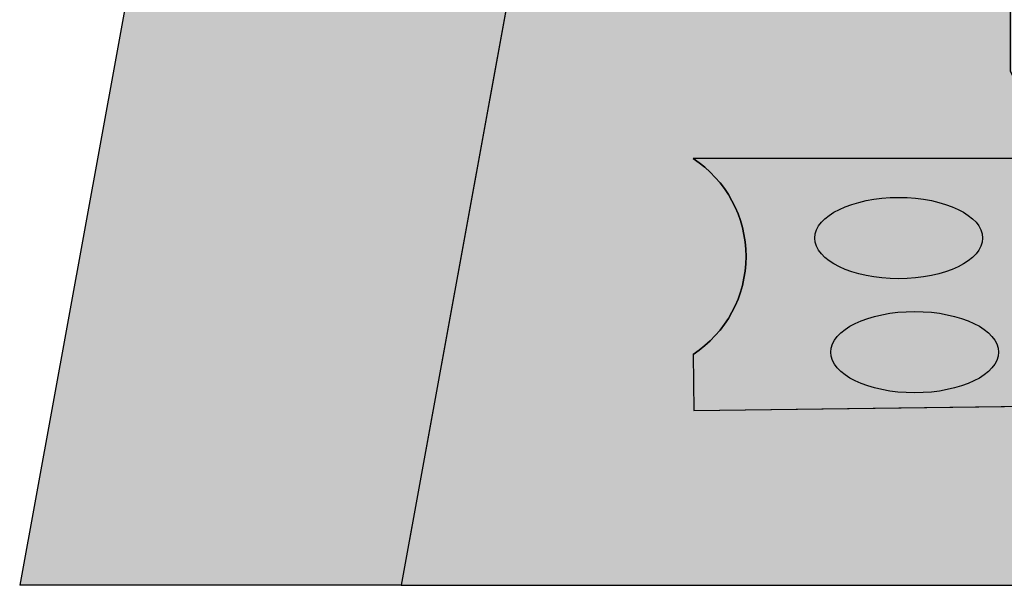
# Model space of a CAD drawing. Units: feet. Extents: x 3168 to 4724, y 827 to 1477.
# Tile 1 of 256: x 3168 to 3599, y 827 to 1075. Entities that reach past the tile are written whole.
import ezdxf

# ---------------------------------------------------------------- set-up
doc = ezdxf.new("R2010")
doc.units = ezdxf.units.FT
doc.layers.add('A-ELEV-PATT', color=8, linetype='Continuous', lineweight=13)
doc.layers.add('C-TOPO', color=3, linetype='Continuous', lineweight=25)

msp = doc.modelspace()

# ---------------------------------------------------------------- hatches: boundary and pattern name
at = {"layer": 'A-ELEV-PATT'}
h = msp.add_hatch(color=256, dxfattribs=at)
h.dxf.hatch_style = 1
edge = h.paths.add_edge_path()
edge.add_ellipse((3552.91, 979.22), major_axis=(36.74, 0), ratio=0.484848, start_angle=0, end_angle=360)
edge = h.paths.add_edge_path()
edge.add_ellipse((3559.89, 929.25), major_axis=(36.74, 0), ratio=0.484848, start_angle=0, end_angle=360)
edge = h.paths.add_edge_path()
edge.add_line((3299.32, 1198.61), (3479.92, 1198.61))
edge.add_line((3479.92, 1198.61), (3479.92, 1209.87))
edge.add_spline(control_points=[(3479.92, 1209.87), (3464.3, 1209.87), (3448.69, 1209.87), (3410.95, 1209.87), (3388.83, 1209.87), (3355.65, 1209.87), (3344.59, 1209.87), (3328, 1209.87), (3322.47, 1209.87), (3314.17, 1209.87), (3311.41, 1209.87), (3307.26, 1209.87), (3305.87, 1209.87), (3303.8, 1209.87), (3303.11, 1209.87), (3302.07, 1209.87), (3301.73, 1209.87), (3301.21, 1209.87), (3301.04, 1209.87), (3300.78, 1209.87), (3300.69, 1209.87), (3300.56, 1209.87), (3300.52, 1209.87), (3300.45, 1209.87), (3300.43, 1209.87), (3300.4, 1209.87), (3300.39, 1209.87), (3300.37, 1209.87), (3300.35, 1209.87), (3300.35, 1209.87), (3300.35, 1209.87), (3300.34, 1209.87), (3300.34, 1209.87), (3300.34, 1209.87), (3300.34, 1209.87), (3300.33, 1209.87), (3300.33, 1209.87), (3300.33, 1209.87), (3300.32, 1209.87), (3300.31, 1209.87), (3300.31, 1209.87), (3300.29, 1209.87), (3300.28, 1209.87), (3300.23, 1209.87), (3300.2, 1209.87), (3299.95, 1209.87), (3299.74, 1209.87), (3299.44, 1209.88), (3299.33, 1209.89), (3299.18, 1209.89), (3299.13, 1209.9), (3298.65, 1209.92), (3298.23, 1209.95), (3297.6, 1210), (3297.39, 1210.02), (3297.08, 1210.06), (3296.98, 1210.07), (3296.29, 1210.15), (3295.72, 1210.24), (3294.87, 1210.4), (3294.59, 1210.45), (3294.17, 1210.54), (3294.03, 1210.57), (3291.71, 1211.1), (3289.65, 1211.81), (3285.78, 1213.56), (3283.95, 1214.6), (3280.51, 1216.98), (3278.9, 1218.32), (3276.38, 1220.83), (3275.42, 1221.92), (3274.04, 1223.71), (3273.58, 1224.35), (3273.14, 1225.02)], knot_values=[39.119033, 39.119033, 39.119033, 39.119033, 39.286353, 39.286353, 39.523379, 39.523379, 39.641892, 39.641892, 39.701148, 39.701148, 39.730777, 39.730777, 39.745591, 39.745591, 39.752998, 39.752998, 39.756701, 39.756701, 39.758553, 39.758553, 39.759479, 39.759479, 39.759942, 39.759942, 39.760173, 39.760173, 39.760289, 39.760289, 39.760405, 39.760405, 39.760463, 39.760463, 39.763389, 39.763389, 39.764851, 39.764851, 39.767304, 39.767304, 39.773825, 39.773825, 39.78057, 39.78057, 39.79477, 39.79477, 39.845194, 39.845194, 40.126715, 40.126715, 40.267476, 40.267476, 40.337856, 40.337856, 40.927023, 40.927023, 41.221606, 41.221606, 41.368898, 41.368898, 42.202622, 42.202622, 42.619485, 42.619485, 42.827916, 42.827916, 46.118323, 46.118323, 49.408731, 49.408731, 52.699139, 52.699139, 54.927489, 54.927489, 56.104228, 56.104228, 56.104228, 56.104228], weights=[1, 1, 1, 1, 1, 1, 1, 1, 1, 1, 1, 1, 1, 1, 1, 1, 1, 1, 1, 1, 1, 1, 1, 1, 1, 1, 1, 1, 1, 1, 1, 1, 1, 1, 1, 1, 1, 1, 1, 1, 1, 1, 1, 1, 1, 1, 1, 1, 1, 1, 1, 1, 1, 1, 1, 1, 1, 1, 1, 1, 1, 1, 1, 1, 1, 1, 1, 1, 1, 1, 1, 1, 1, 1], degree=3, periodic=0)
edge.add_line((3273.14, 1225.02), (3273.14, 1099.02))
edge.add_line((3273.14, 1099.02), (3299.32, 1099.02))
edge.add_line((3299.32, 1099.02), (3299.32, 1198.61))
edge = h.paths.add_edge_path()
edge.add_line((3304.76, 1324.16), (3479.92, 1324.16))
edge.add_line((3479.92, 1324.16), (3479.92, 1335.71))
edge.add_line((3479.92, 1335.71), (3269.16, 1335.71))
edge.add_spline(control_points=[(3269.16, 1335.71), (3264.02, 1335.71), (3258.36, 1328.96), (3259.26, 1323.9)], knot_values=[0, 0, 0, 0, 15.412191, 15.412191, 15.412191, 15.412191], degree=3, periodic=0)
edge.add_line((3259.26, 1323.9), (3265.52, 1288.77))
edge.add_line((3265.52, 1288.77), (3275.27, 1261.55))
edge.add_line((3275.27, 1261.55), (3304.76, 1261.55))
edge.add_line((3304.76, 1261.55), (3304.76, 1324.16))
h = msp.add_hatch(color=256, dxfattribs=at)
h.dxf.hatch_style = 1
h.paths.add_polyline_path([(3384.53, 1099.02), (3335.03, 1099.02), (3299.32, 1099.02), (3273.14, 1099.02), (3217.57, 1099.02), (3168.07, 827.12), (3335.03, 827.12)])
h = msp.add_hatch(color=256, dxfattribs=at)
h.dxf.hatch_style = 1
h.paths.add_polyline_path([(3845.38, 1099.02), (3706.29, 1099.02), (3715.62, 1081.4), (3715.62, 1052.31), (3792.06, 907.96), (3463.22, 903.64), (3462.9, 928.26, 0.540152), (3462.9, 1014.08), (3621.9, 1014.08), (3601.66, 1052.31), (3601.66, 1081.4), (3592.33, 1099.02), (3384.53, 1099.02), (3335.03, 827.12), (3845.38, 827.12)])
h = msp.add_hatch(color=256, dxfattribs=at)
h.dxf.hatch_style = 1
h.paths.add_polyline_path([(3715.62, 1052.31), (3715.62, 1081.4), (3706.29, 1099.02), (3592.33, 1099.02), (3601.66, 1081.4), (3601.66, 1052.31), (3621.9, 1014.08), (3462.9, 1014.08, -0.540152), (3462.9, 928.26), (3463.22, 903.64), (3792.06, 907.96)])
edge = h.paths.add_edge_path(flags=16)
edge.add_ellipse((3559.89, 929.25), major_axis=(36.74, 0), ratio=0.484848, start_angle=0, end_angle=360)
edge = h.paths.add_edge_path(flags=16)
edge.add_ellipse((3552.91, 979.22), major_axis=(36.74, 0), ratio=0.484848, start_angle=0, end_angle=360)

# ---------------------------------------------------------------- linework, layer by layer
at = {"layer": 'C-TOPO'}
for p, q in [((3384.53, 1099.02), (3335.03, 827.12)), ((3621.9, 1014.08), (3462.9, 1014.08)), ((3462.9, 928.26), (3463.22, 903.64)), ((3463.22, 903.64), (3792.06, 907.96)), ((3335.03, 827.12), (3168.07, 827.12))]:
    msp.add_line(p, q, dxfattribs=at)
for points in [[(3217.57, 1099.02), (3168.07, 827.12)], [(3384.53, 1099.02), (3335.03, 827.12), (3845.38, 827.12), (3845.38, 1099.02), (3335.03, 1099.02)], [(3335.03, 827.12), (3845.38, 827.12), (3845.38, 1099.02), (3335.03, 1099.02)]]:
    msp.add_lwpolyline(points, dxfattribs=at)
msp.add_lwpolyline([(3592.33, 1099.02), (3601.66, 1081.4), (3601.66, 1052.31), (3621.9, 1014.08), (3462.9, 1014.08, -0.540152), (3462.9, 928.26), (3463.22, 903.64), (3792.06, 907.96), (3715.62, 1052.31), (3715.62, 1081.4), (3706.29, 1099.02)], format="xyb", dxfattribs=at)
msp.add_arc((3434.77, 971.17), 51.31, 303.2484, 56.7516, dxfattribs=at)
for centre in [(3552.91, 979.22), (3552.91, 979.22), (3559.89, 929.25), (3559.89, 929.25)]:
    msp.add_ellipse(centre, major_axis=(36.74, 0), ratio=0.484848, dxfattribs=at)

doc.saveas('drawing.dxf')
